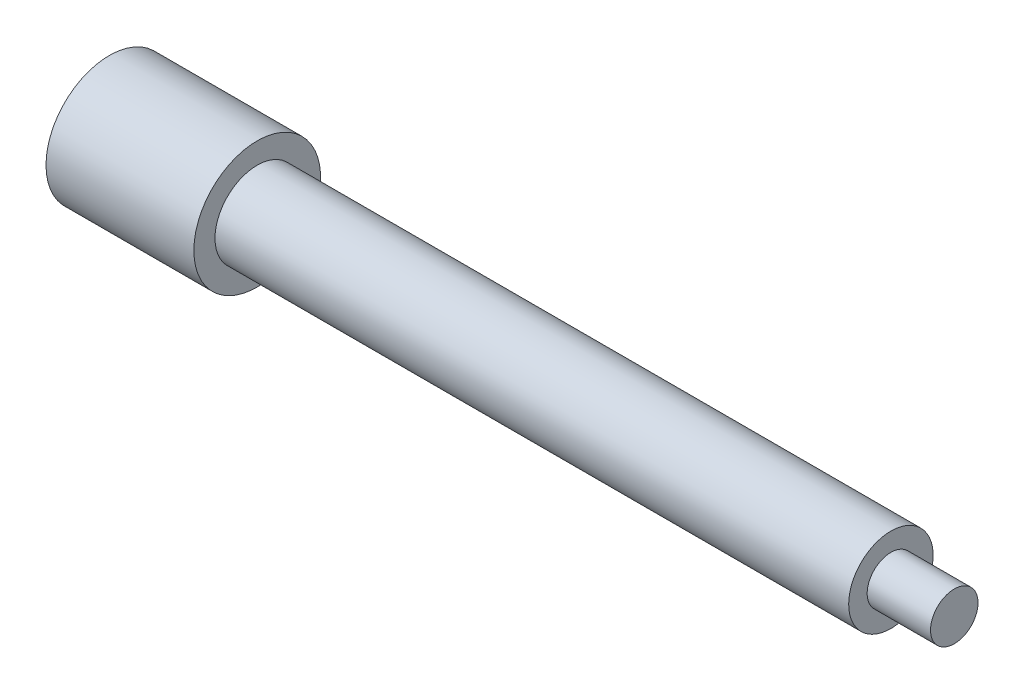
ISO-10303-21;
HEADER;
FILE_DESCRIPTION(('STEP AP214'),'2;1');
FILE_NAME('part.step','',(''),(''),'','','');
FILE_SCHEMA(('AUTOMOTIVE_DESIGN { 1 0 10303 214 1 1 1 1 }'));
ENDSEC;
DATA;
#1=APPLICATION_CONTEXT('core data for automotive mechanical design processes');
#2=APPLICATION_PROTOCOL_DEFINITION('international standard','automotive_design',2000,#1);
#3=PRODUCT_CONTEXT('',#1,'mechanical');
#4=PRODUCT('Part','Part','',(#3));
#5=PRODUCT_RELATED_PRODUCT_CATEGORY('part','',(#4));
#6=PRODUCT_DEFINITION_FORMATION('','',#4);
#7=PRODUCT_DEFINITION_CONTEXT('part definition',#1,'design');
#8=PRODUCT_DEFINITION('design','',#6,#7);
#9=PRODUCT_DEFINITION_SHAPE('','',#8);
#10=(LENGTH_UNIT() NAMED_UNIT(*) SI_UNIT(.MILLI.,.METRE.));
#11=(NAMED_UNIT(*) PLANE_ANGLE_UNIT() SI_UNIT($,.RADIAN.));
#12=(NAMED_UNIT(*) SI_UNIT($,.STERADIAN.) SOLID_ANGLE_UNIT());
#13=UNCERTAINTY_MEASURE_WITH_UNIT(LENGTH_MEASURE(1.E-05),#10,'distance_accuracy_value','');
#14=(GEOMETRIC_REPRESENTATION_CONTEXT(3) GLOBAL_UNCERTAINTY_ASSIGNED_CONTEXT((#13)) GLOBAL_UNIT_ASSIGNED_CONTEXT((#10,
#11,#12)) REPRESENTATION_CONTEXT('',''));
#15=CARTESIAN_POINT('',(0.,0.,0.));
#16=DIRECTION('',(0.,0.,1.));
#17=DIRECTION('',(1.,0.,0.));
#18=AXIS2_PLACEMENT_3D('',#15,#16,#17);
#19=CARTESIAN_POINT('',(0.,0.,0.));
#20=DIRECTION('',(1.,0.,0.));
#21=DIRECTION('',(0.,0.,-1.));
#22=AXIS2_PLACEMENT_3D('',#19,#20,#21);
#23=PLANE('',#22);
#24=CARTESIAN_POINT('',(0.,0.,0.));
#25=DIRECTION('',(-1.,0.,0.));
#26=DIRECTION('',(0.,0.,1.));
#27=AXIS2_PLACEMENT_3D('',#24,#25,#26);
#28=CIRCLE('',#27,6.);
#29=CARTESIAN_POINT('',(0.,0.,6.));
#30=VERTEX_POINT('',#29);
#31=EDGE_CURVE('E10',#30,#30,#28,.T.);
#32=ORIENTED_EDGE('',*,*,#31,.T.);
#33=EDGE_LOOP('',(#32));
#34=FACE_BOUND('',#33,.T.);
#35=ADVANCED_FACE('F40',(#34),#23,.F.);
#36=CARTESIAN_POINT('',(0.,0.,0.));
#37=DIRECTION('',(-1.,0.,0.));
#38=DIRECTION('',(0.,0.,1.));
#39=AXIS2_PLACEMENT_3D('',#36,#37,#38);
#40=CYLINDRICAL_SURFACE('',#39,6.);
#41=ORIENTED_EDGE('',*,*,#31,.F.);
#42=EDGE_LOOP('',(#41));
#43=FACE_BOUND('',#42,.T.);
#44=CARTESIAN_POINT('',(14.,0.,0.));
#45=DIRECTION('',(-1.,0.,0.));
#46=DIRECTION('',(0.,0.,1.));
#47=AXIS2_PLACEMENT_3D('',#44,#45,#46);
#48=CIRCLE('',#47,6.);
#49=CARTESIAN_POINT('',(14.,0.,6.));
#50=VERTEX_POINT('',#49);
#51=EDGE_CURVE('E43',#50,#50,#48,.T.);
#52=ORIENTED_EDGE('',*,*,#51,.T.);
#53=EDGE_LOOP('',(#52));
#54=FACE_BOUND('',#53,.T.);
#55=ADVANCED_FACE('F73',(#43,#54),#40,.T.);
#56=CARTESIAN_POINT('',(14.,6.,0.));
#57=DIRECTION('',(-1.,0.,0.));
#58=DIRECTION('',(0.,0.,1.));
#59=AXIS2_PLACEMENT_3D('',#56,#57,#58);
#60=PLANE('',#59);
#61=ORIENTED_EDGE('',*,*,#51,.F.);
#62=EDGE_LOOP('',(#61));
#63=FACE_BOUND('',#62,.T.);
#64=CARTESIAN_POINT('',(14.,0.,0.));
#65=DIRECTION('',(-1.,0.,0.));
#66=DIRECTION('',(0.,0.,1.));
#67=AXIS2_PLACEMENT_3D('',#64,#65,#66);
#68=CIRCLE('',#67,4.);
#69=CARTESIAN_POINT('',(14.,0.,4.));
#70=VERTEX_POINT('',#69);
#71=EDGE_CURVE('E50',#70,#70,#68,.T.);
#72=ORIENTED_EDGE('',*,*,#71,.T.);
#73=EDGE_LOOP('',(#72));
#74=FACE_BOUND('',#73,.T.);
#75=ADVANCED_FACE('F80',(#63,#74),#60,.F.);
#76=CARTESIAN_POINT('',(0.,0.,0.));
#77=DIRECTION('',(-1.,0.,0.));
#78=DIRECTION('',(0.,0.,1.));
#79=AXIS2_PLACEMENT_3D('',#76,#77,#78);
#80=CYLINDRICAL_SURFACE('',#79,4.);
#81=ORIENTED_EDGE('',*,*,#71,.F.);
#82=EDGE_LOOP('',(#81));
#83=FACE_BOUND('',#82,.T.);
#84=CARTESIAN_POINT('',(74.,0.,0.));
#85=DIRECTION('',(-1.,0.,0.));
#86=DIRECTION('',(0.,0.,1.));
#87=AXIS2_PLACEMENT_3D('',#84,#85,#86);
#88=CIRCLE('',#87,4.);
#89=CARTESIAN_POINT('',(74.,0.,4.));
#90=VERTEX_POINT('',#89);
#91=EDGE_CURVE('E51',#90,#90,#88,.T.);
#92=ORIENTED_EDGE('',*,*,#91,.T.);
#93=EDGE_LOOP('',(#92));
#94=FACE_BOUND('',#93,.T.);
#95=ADVANCED_FACE('F82',(#83,#94),#80,.T.);
#96=CARTESIAN_POINT('',(74.,4.,0.));
#97=DIRECTION('',(-1.,0.,0.));
#98=DIRECTION('',(0.,0.,1.));
#99=AXIS2_PLACEMENT_3D('',#96,#97,#98);
#100=PLANE('',#99);
#101=ORIENTED_EDGE('',*,*,#91,.F.);
#102=EDGE_LOOP('',(#101));
#103=FACE_BOUND('',#102,.T.);
#104=CARTESIAN_POINT('',(74.,0.,0.));
#105=DIRECTION('',(-1.,0.,0.));
#106=DIRECTION('',(0.,0.,1.));
#107=AXIS2_PLACEMENT_3D('',#104,#105,#106);
#108=CIRCLE('',#107,2.25);
#109=CARTESIAN_POINT('',(74.,0.,2.25));
#110=VERTEX_POINT('',#109);
#111=EDGE_CURVE('E57',#110,#110,#108,.T.);
#112=ORIENTED_EDGE('',*,*,#111,.T.);
#113=EDGE_LOOP('',(#112));
#114=FACE_BOUND('',#113,.T.);
#115=ADVANCED_FACE('F72',(#103,#114),#100,.F.);
#116=CARTESIAN_POINT('',(0.,0.,0.));
#117=DIRECTION('',(-1.,0.,0.));
#118=DIRECTION('',(0.,0.,1.));
#119=AXIS2_PLACEMENT_3D('',#116,#117,#118);
#120=CYLINDRICAL_SURFACE('',#119,2.25);
#121=ORIENTED_EDGE('',*,*,#111,.F.);
#122=EDGE_LOOP('',(#121));
#123=FACE_BOUND('',#122,.T.);
#124=CARTESIAN_POINT('',(80.,0.,0.));
#125=DIRECTION('',(-1.,0.,0.));
#126=DIRECTION('',(0.,0.,1.));
#127=AXIS2_PLACEMENT_3D('',#124,#125,#126);
#128=CIRCLE('',#127,2.25);
#129=CARTESIAN_POINT('',(80.,0.,2.25));
#130=VERTEX_POINT('',#129);
#131=EDGE_CURVE('E56',#130,#130,#128,.T.);
#132=ORIENTED_EDGE('',*,*,#131,.T.);
#133=EDGE_LOOP('',(#132));
#134=FACE_BOUND('',#133,.T.);
#135=ADVANCED_FACE('F62',(#123,#134),#120,.T.);
#136=CARTESIAN_POINT('',(80.,2.25,0.));
#137=DIRECTION('',(-1.,0.,0.));
#138=DIRECTION('',(0.,0.,1.));
#139=AXIS2_PLACEMENT_3D('',#136,#137,#138);
#140=PLANE('',#139);
#141=ORIENTED_EDGE('',*,*,#131,.F.);
#142=EDGE_LOOP('',(#141));
#143=FACE_BOUND('',#142,.T.);
#144=ADVANCED_FACE('F61',(#143),#140,.F.);
#145=CLOSED_SHELL('',(#35,#55,#75,#95,#115,#135,#144));
#146=MANIFOLD_SOLID_BREP('B2',#145);
#147=ADVANCED_BREP_SHAPE_REPRESENTATION('',(#18,#146),#14);
#148=SHAPE_DEFINITION_REPRESENTATION(#9,#147);
ENDSEC;
END-ISO-10303-21;
